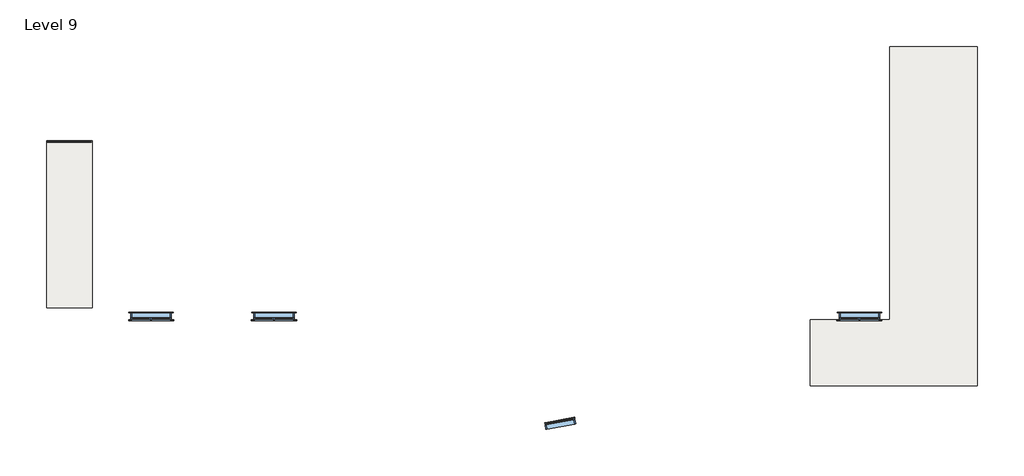
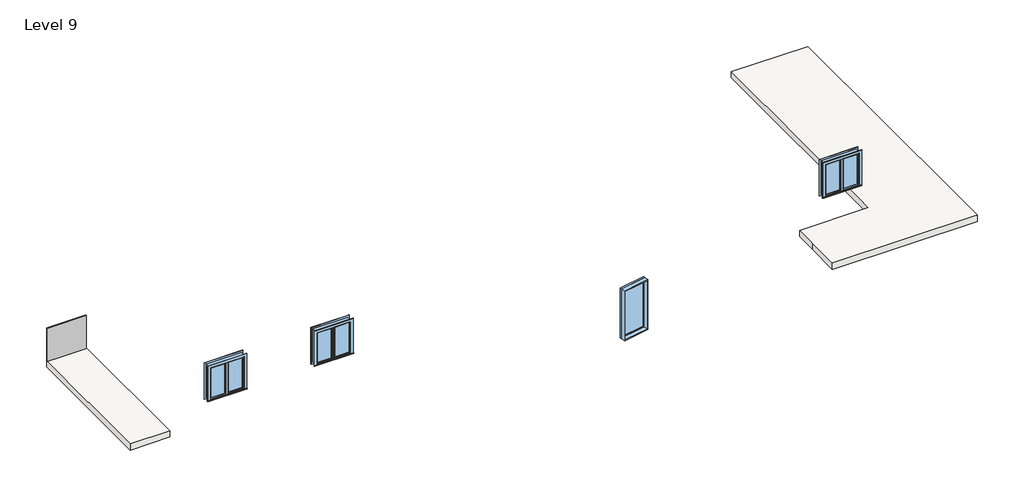
# One storey: 4 windows, 2 slabs, 1 plate.
"""IFC4 building model written with IfcOpenShell, lengths in millimetres."""

from ifc_helpers import new_model, si_unit, frame, origin, place, context, project, spatial, polyline, outline, extrude, transform, mapped, element, save
from components import system_panel_glazed_7d767388, window_0862ab64, window_9a779fa2

model = new_model("IFC4")

# Units and contexts
model_context = context("Model", 3, world=origin())
ifc_project = project(units=[si_unit("LENGTHUNIT", "METRE", prefix="MILLI")], contexts=[model_context])

# Site, building, storey
site = spatial("IfcSite", under=ifc_project)
building = spatial("IfcBuilding", under=site)
storey = spatial("IfcBuildingStorey", under=building, Name="Level 9", Elevation=13106.4)

# Plate
placement = place(None, origin())
system_panel_glazed_shape = system_panel_glazed_7d767388(model_context)
element("IfcPlate", 1, ObjectType="System Panel : Glazed", at=placement, inside=storey, context=model_context, shape_type="MappedRepresentation", body=[
    mapped(system_panel_glazed_shape, transform((-17306.4505427, -8690.0239591, 13106.4), x_axis=(-1.0, 0.0, 0.0), y_axis=(0.0, -1.0, 0.0), z_axis=(0.0, 0.0, 1.0))),
])

# Slabs
element("IfcSlab", 2, ObjectType="9\"", at=placement, inside=storey, context=model_context, shape_type="SweptSolid", body=[
    extrude(outline(polyline([(-17979.5505427, -8690.0239591), (-16607.9505427, -8690.0239591), (-16607.9505427, -13719.2239591), (-17979.5505427, -13719.2239591), (-17979.5505427, -8690.0239591)])), frame((0.0, 0.0, 12877.8), z_axis=(0.0, 0.0, 1.0), x_axis=(1.0, 0.0, 0.0)), (0.0, 0.0, 1.0), 228.6),
])
element("IfcSlab", 3, ObjectType="9\"", at=placement, inside=storey, context=model_context, shape_type="SweptSolid", body=[
    extrude(outline(polyline([(5032.8494573, -14840.0808221), (5032.8494573, -14078.0808221), (7217.2494573, -14078.0808221), (7420.4494573, -14078.0808221), (7420.4494573, -5848.4808221), (10062.0494573, -5848.4808221), (10062.0494573, -14840.0808221), (10062.0494573, -16059.2808221), (5032.8494573, -16059.2808221), (5032.8494573, -14840.0808221)])), frame((0.0, 0.0, 12877.8), z_axis=(0.0, 0.0, 1.0), x_axis=(1.0, 0.0, 0.0)), (0.0, 0.0, 1.0), 228.6),
])

# Windows
window_shape = window_0862ab64(model_context)
element("IfcWindow", 4, ObjectType="Casement Dbl with Trim : 48\" x 48\"", at=placement, inside=storey, context=model_context, shape_type="MappedRepresentation", body=[
    mapped(window_shape, transform((-11129.6382271, -13957.4308221, 13106.4), x_axis=(-1.0, 0.0, 0.0), y_axis=(0.0, -1.0, 0.0), z_axis=(0.0, 0.0, 1.0))),
])
element("IfcWindow", 5, ObjectType="Casement Dbl with Trim : 48\" x 48\"", at=placement, inside=storey, context=model_context, shape_type="MappedRepresentation", body=[
    mapped(window_shape, transform((-14829.9505427, -13957.4308221, 13106.4), x_axis=(-1.0, 0.0, 0.0), y_axis=(0.0, -1.0, 0.0), z_axis=(0.0, 0.0, 1.0))),
])
element("IfcWindow", 6, ObjectType="Casement Dbl with Trim : 48\" x 48\"", at=placement, inside=storey, context=model_context, shape_type="MappedRepresentation", body=[
    mapped(window_shape, transform((6506.0494573, -13957.4308221, 13106.4), x_axis=(-1.0, 0.0, 0.0), y_axis=(0.0, -1.0, 0.0), z_axis=(0.0, 0.0, 1.0))),
])
window_2_shape = window_9a779fa2(model_context)
element("IfcWindow", 7, ObjectType="Fixed : 36\" x 72\"", at=placement, inside=storey, context=model_context, shape_type="MappedRepresentation", body=[
    mapped(window_2_shape, transform((-2469.9901523, -17191.5852128, 13543.6158009), x_axis=(0.9843456980765536, 0.17624853666961993, 0.0), y_axis=(-0.17624853666961993, 0.9843456980765536, 0.0), z_axis=(0.0, 0.0, 1.0))),
])

save(model, "model.ifc")

# Revit data of these elements
# Type "System Panel : Glazed"
#   Construction Type Id = "GSP4R"
#   Analytic Construction = "1/8 in Pilkington single glazing"
#   Visual Light Transmittance = 0.9
#   Solar Heat Gain Coefficient = 0.86
#   Heat Transfer Coefficient (U) = 1.18115 BTU/(h·ft²·°F)
# Type "9\""
#   Assembly Code = "B1010"
#   Function = 0
#   Layers, outside or top first: 0' - 9" no material (function 1)
# Type "Casement Dbl with Trim : 48\" x 48\""
#   Type Mark = "10"
#   Construction Type Id = "GSP4R"
#   Assembly Code = "B2020100"
#   Analytic Construction = "1/8 in Pilkington single glazing"
#   Visual Light Transmittance = 0.9
#   Solar Heat Gain Coefficient = 0.78
#   Heat Transfer Coefficient (U) = 0.6496 BTU/(h·ft²·°F)
#   Height = 4' - 0"
#   Default Sill Height = 3' - 0"
#   Trim Projection - Ext. = 0' - 0 1/2"
#   Trim Projection - Int. = 0' - 0 3/4"
#   Trim Width - Exterior = 0' - 3 1/2"
#   Trim Width - Interior = 0' - 3 1/2"
#   Width = 4' - 0"
#   Window Inset = 0' - 0 3/4"
#   Define Thermal Properties by = 1
#   Glass Pane Material = Glass
#   Sash Material = Sash
#   Trim Exterior Material = Trim
#   Trim Interior Material = Trim
#   Wall Closure = (empty or 0)
# Type "Fixed : 36\" x 72\""
#   Type Mark = "9"
#   Construction Type Id = "GSP4R"
#   Assembly Code = "B2020100"
#   Analytic Construction = "1/8 in Pilkington single glazing"
#   Visual Light Transmittance = 0.9
#   Solar Heat Gain Coefficient = 0.78
#   Heat Transfer Coefficient (U) = 0.6496 BTU/(h·ft²·°F)
#   Height = 6' - 0"
#   Default Sill Height = 1' - 0"
#   Width = 3' - 0"
#   Window Inset = 0' - 0 3/4"
#   Define Thermal Properties by = 1
#   Glass Pane Material = Glass
#   Sash Material = Sash
#   Wall Closure = (empty or 0)
# Element 1 (IfcPlate, "System Panel : Glazed")
#   Phase Created = New Construction
#   Materials on its faces: "Glass"
# Element 2 (IfcSlab, "9\"")
#   built-in parameter 1001955 = 3.14159 (stored number, unit not read)
#   Height Offset From Level = 0' - 0"
#   Phase Created = New Construction
#   Materials on its faces: "Default Floor"
# Element 3 (IfcSlab, "9\"")
#   built-in parameter 1001955 = -1.5708 (stored number, unit not read)
#   Height Offset From Level = 0' - 0"
#   Phase Created = New Construction
#   Materials on its faces: "Default Floor"
# Element 4 (IfcWindow, "Casement Dbl with Trim : 48\" x 48\"")
#   Mark = "39"
#   Phase Created = New Construction
#   Materials on its faces: "Sash", "Trim", "Glass"
# Element 5 (IfcWindow, "Casement Dbl with Trim : 48\" x 48\"")
#   Mark = "40"
#   Phase Created = New Construction
#   Materials on its faces: "Sash", "Trim", "Glass"
# Element 6 (IfcWindow, "Casement Dbl with Trim : 48\" x 48\"")
#   Mark = "57"
#   Phase Created = New Construction
#   Materials on its faces: "Sash", "Trim", "Glass"
# Element 7 (IfcWindow, "Fixed : 36\" x 72\"")
#   Mark = "12"
#   Phase Created = New Construction
#   Materials on its faces: "Sash", "Glass"
# Materials
#   "Glass": class "Glass", colour RGB 0 128 192, transparency 0.75, Description = "Soda Lime Glass", Cost = 0
#   "Sash": class "Wood", colour RGB 224 178 126, transparency 0
#   "Trim": class "Wood", colour RGB 224 178 126, transparency 0
#   "Default Floor": colour RGB 128 128 128, transparency 0
